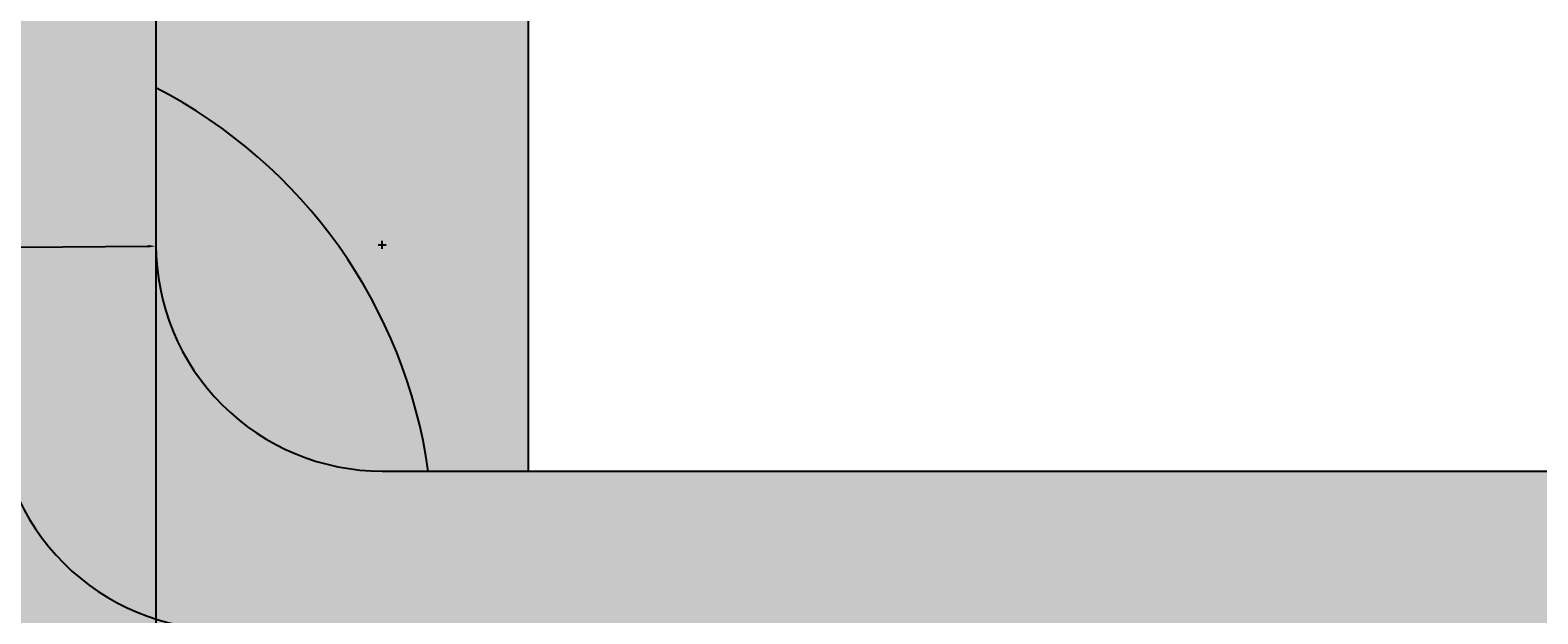
# Model space of a CAD drawing. Units: millimetres. Extents: x -11 to 280, y -4 to 208.
# Tile 33 of 55: x 189 to 222, y 76 to 88. Entities that reach past the tile are written whole.
import ezdxf

# ---------------------------------------------------------------- set-up
doc = ezdxf.new("R2010")
doc.units = ezdxf.units.MM
for name, color, linetype, lineweight in [('M-DIMS', 2, 'Continuous', 18), ('M-HYDR-PRES', 7, 'Continuous', 25), ('M-HYDR-VALV', 7, 'Continuous', 25), ('M-HYDR-VALV-PATT', 252, 'Continuous', 13)]:
    doc.layers.add(name, color=color, linetype=linetype, lineweight=lineweight)
doc.layers.add('M-HYDR-PRES-PATT', color=240, linetype='Continuous', lineweight=13, true_color=0xed1f24)
doc.styles.get("Standard").update_dxf_attribs({"font": 'arial.ttf'})
doc.dimstyles.get("Standard").update_dxf_attribs({"dimtxt": 0.18, "dimasz": 0.18, "dimexe": 0.18, "dimexo": 0.0625, "dimgap": 0.09, "dimtad": 0, "dimtih": 1, "dimtoh": 1, "dimdec": 4, "dimzin": 0, "dimdsep": 46, "dimtxsty": 'Standard', "dimcen": 0.09, "dimadec": 0, "dimazin": 0, "dimtfac": 1, "dimtdec": 4, "dimtofl": 0, "dimtmove": 0, "dimatfit": 3, "dimfxl": 1, "dimtolj": 1, "dimtzin": 0, "dimarcsym": 0})

# ---------------------------------------------------------------- blocks, each defined once
blk = doc.blocks.new('*D4')
at = {"layer": 'Defpoints', "color": 0, "transparency": 16777216}
for p in [(4.763, 84.426), (266.035, 51.733), (266.035, -3.415)]:
    blk.add_point(p, dxfattribs=at)
at = {"layer": 'M-DIMS', "color": 0, "lineweight": -2, "transparency": 16777216}
for p, q in [((4.763, 84.364), (4.763, -3.595)), ((266.035, 51.67), (266.035, -3.595)), ((4.943, -3.415), (134.934, -3.415)), ((265.855, -3.415), (135.864, -3.415))]:
    blk.add_line(p, q, dxfattribs=at)
at = {"layer": 'M-DIMS', "color": 0, "transparency": 16777216}
for points in [[(4.943, -3.385), (4.943, -3.445), (4.763, -3.415)], [(265.855, -3.385), (265.855, -3.445), (266.035, -3.415)]]:
    blk.add_solid(points, dxfattribs=at)
at = {"layer": 'M-DIMS', "color": 0, "transparency": 16777216, "insert": (135.399, -3.415), "char_height": 0.18, "attachment_point": 5}
blk.add_mtext('\\A1;261.27', dxfattribs=at)
blk = doc.blocks.new('*D5')
at = {"layer": 'Defpoints', "color": 0, "transparency": 16777216}
for p in [(24.759, 192.645), (-10.087, 11.435), (261.686, 11.435)]:
    blk.add_point(p, dxfattribs=at)
at = {"layer": 'M-DIMS', "color": 0, "lineweight": -2, "transparency": 16777216}
for p, q in [((24.696, 192.645), (-10.267, 192.645)), ((-10.087, 192.465), (-10.087, 102.222)), ((-10.087, 11.615), (-10.087, 101.858)), ((261.624, 11.435), (-10.267, 11.435))]:
    blk.add_line(p, q, dxfattribs=at)
at = {"layer": 'M-DIMS', "color": 0, "transparency": 16777216}
for points in [[(-10.117, 192.465), (-10.057, 192.465), (-10.087, 192.645)], [(-10.117, 11.615), (-10.057, 11.615), (-10.087, 11.435)]]:
    blk.add_solid(points, dxfattribs=at)
at = {"layer": 'M-DIMS', "color": 0, "transparency": 16777216, "insert": (-10.087, 102.04), "char_height": 0.18, "attachment_point": 5}
blk.add_mtext('\\A1;181.2', dxfattribs=at)
blk = doc.blocks.new('*D13')
at = {"layer": 'Defpoints', "color": 0, "transparency": 16777216}
for p in [(191.774, 105.314), (232.2, 105.314), (232.2, -3.415)]:
    blk.add_point(p, dxfattribs=at)
at = {"layer": 'M-DIMS', "color": 0, "lineweight": -2, "transparency": 16777216}
for p, q in [((191.774, 105.252), (191.774, -3.595)), ((232.2, 105.252), (232.2, -3.595)), ((191.954, -3.415), (211.52, -3.415)), ((232.02, -3.415), (212.454, -3.415))]:
    blk.add_line(p, q, dxfattribs=at)
at = {"layer": 'M-DIMS', "color": 0, "transparency": 16777216}
for points in [[(191.954, -3.385), (191.954, -3.445), (191.774, -3.415)], [(232.02, -3.385), (232.02, -3.445), (232.2, -3.415)]]:
    blk.add_solid(points, dxfattribs=at)
at = {"layer": 'M-DIMS', "color": 0, "transparency": 16777216, "insert": (211.987, -3.415), "char_height": 0.18, "attachment_point": 5}
blk.add_mtext('\\A1;40.426', dxfattribs=at)
blk = doc.blocks.new('*D20')
at = {"layer": 'Defpoints', "color": 0, "transparency": 16777216}
for p in [(231.68, 207.495), (151.022, 43.599), (231.68, 43.599)]:
    blk.add_point(p, dxfattribs=at)
at = {"layer": 'M-DIMS', "color": 0, "lineweight": -2, "transparency": 16777216}
for p, q in [((151.022, 43.662), (151.022, 207.675)), ((231.68, 43.662), (231.68, 207.675)), ((151.202, 207.495), (190.957, 207.495)), ((231.5, 207.495), (191.745, 207.495))]:
    blk.add_line(p, q, dxfattribs=at)
at = {"layer": 'M-DIMS', "color": 0, "transparency": 16777216}
for points in [[(151.202, 207.525), (151.202, 207.465), (151.022, 207.495)], [(231.5, 207.525), (231.5, 207.465), (231.68, 207.495)]]:
    blk.add_solid(points, dxfattribs=at)
at = {"layer": 'M-DIMS', "color": 0, "transparency": 16777216, "insert": (191.351, 207.495), "char_height": 0.18, "attachment_point": 5}
blk.add_mtext('\\A1;80.66', dxfattribs=at)
blk = doc.blocks.new('*D31')
at = {"layer": 'Defpoints', "color": 0, "transparency": 16777216}
for p in [(191.775, 83.68), (196.774, 83.71)]:
    blk.add_point(p, dxfattribs=at)
at = {"layer": 'M-DIMS', "color": 0, "lineweight": -2, "transparency": 16777216}
for p, q in [((188.775, 83.662), (191.595, 83.679)), ((196.684, 83.71), (196.864, 83.71)), ((196.774, 83.62), (196.774, 83.8))]:
    blk.add_line(p, q, dxfattribs=at)
at = {"layer": 'M-DIMS', "color": 0, "transparency": 16777216}
blk.add_solid([(191.594, 83.709), (191.595, 83.649), (191.775, 83.68)], dxfattribs=at)
at = {"layer": 'M-DIMS', "color": 0, "transparency": 16777216, "insert": (188.342, 83.662), "char_height": 0.18, "attachment_point": 5}
blk.add_mtext('\\A1;4X R5', dxfattribs=at)

msp = doc.modelspace()

# ---------------------------------------------------------------- hatches: boundary and pattern name
at = {"layer": 'M-HYDR-PRES-PATT'}
h = msp.add_hatch(color=256, dxfattribs=at)
h.set_gradient(color1=(237, 31, 36), color2=(237, 31, 36), tint=1)
h.paths.add_polyline_path([(232.2, 133.1228), (228.7, 133.1228), (228.7, 108.8141), (102.7646, 108.8141), (102.7646, 105.3141), (232.2, 105.3141)])
h.paths.add_polyline_path([(128.8433, 105.3141), (125.3433, 105.3141), (125.3433, 91.7099, 1), (128.8433, 91.7099)])
h.paths.add_polyline_path([(229.1617, 78.7098), (196.7745, 78.7098, -0.4142136), (191.7745, 83.7098), (191.7745, 105.3141), (188.2745, 105.3141), (188.2745, 80.2098, 0.4142136), (193.2745, 75.2098), (225.6617, 75.2098), (225.6617, 43.5991), (229.1617, 43.5991)])
h.paths.add_polyline_path([(102.7646, 110.3704), (95.5776, 110.3704), (95.5776, 103.9022), (102.7646, 103.9022)])
h.paths.add_polyline_path([(100.7059, 107.2502), (99.1711, 106.3641), (99.1711, 106.8641), (97.1711, 106.8641), (97.1711, 107.6363), (99.1711, 107.6363), (99.1711, 108.1363)], flags=16)
h.paths.add_polyline_path([(234.6119, 138.4081), (226.5106, 138.4081), (226.5106, 133.1228), (234.6119, 133.1228)])
h.paths.add_polyline_path([(231.1963, 135.7055), (230.2965, 134.1786), (229.4241, 135.7213), (229.9241, 135.7168), (229.9418, 137.7167), (230.7141, 137.7099), (230.6963, 135.71)], flags=16)
at = {"layer": 'M-HYDR-VALV-PATT'}
h = msp.add_hatch(color=256, dxfattribs=at)
h.set_gradient(color1=(153, 27, 30), color2=(153, 27, 30), tint=1)
h.paths.add_polyline_path([(131.8437, 88.2421, -0.3394543), (132.5849, 89.208), (121.2548, 86.1721, -0.4931454), (122.5137, 85.2062, -0.3394543), (121.7725, 84.2403), (133.1025, 87.2762, -0.4931454)])
h.paths.add_polyline_path([(133.1025, 83.1351, -0.4931454), (131.8437, 84.101, -0.3394543), (132.5849, 85.0669), (121.2548, 82.031, -0.4931454), (122.5137, 81.0651, -0.3394543), (121.7725, 80.0992)])
h.paths.add_polyline_path([(133.1025, 78.994, -0.4931454), (131.8437, 79.9599, -0.3394543), (132.5849, 80.9258), (121.2548, 77.8899, -0.4931454), (122.5137, 76.924, -0.3394543), (121.7725, 75.9581)])
h.paths.add_polyline_path([(197.7905, 78.7098), (200.0003, 78.7098), (200.0003, 89.3873), (191.7745, 89.3873), (191.7745, 87.1776, -0.2439164)])
h.paths.add_polyline_path([(200.0003, 65.0638), (200.0003, 75.2098), (197.7325, 75.2098, -0.4135811), (184.7092, 66.0277), (184.7092, 65.0638)])
h.paths.add_polyline_path([(181.2092, 65.0638), (181.2092, 67.2471, -0.2598454), (175.3563, 76.54), (173.8038, 76.54), (173.8038, 65.0638)])
h.paths.add_polyline_path([(188.2745, 88.3022), (188.2745, 89.3873), (173.8038, 89.3873), (173.8038, 80.04), (175.7181, 80.04, -0.3816661)])
h = msp.add_hatch(color=256, dxfattribs=at)
h.set_gradient(color1=(205, 105, 40), color2=(34, 52, 110), tint=1, name='INVCYLINDER')
h.paths.add_polyline_path([(188.2745, 80.2098), (188.2745, 88.3022, 0.3816661), (175.7181, 80.04), (179.7092, 80.04, -0.4142136), (184.7092, 75.04), (184.7092, 66.0277, 0.4135811), (197.7325, 75.2098), (193.2745, 75.2098, -0.4142136)])
h.paths.add_polyline_path([(176.2092, 76.54), (175.3563, 76.54, 0.2598454), (181.2092, 67.2471), (181.2092, 71.54, 0.4142136)])
h.paths.add_polyline_path([(196.7745, 78.7098), (197.7905, 78.7098, 0.2439164), (191.7745, 87.1776), (191.7745, 83.7098, 0.4142136)])

# ---------------------------------------------------------------- linework, layer by layer
at = {"layer": 'M-HYDR-PRES'}
for points in [[(188.2745, 105.3141), (188.2745, 80.2098, 0.4142136), (193.2745, 75.2098), (225.6617, 75.2098), (225.6617, 43.5991)], [(191.7745, 105.3141), (191.7745, 83.7098, 0.4142136), (196.7745, 78.7098), (229.1617, 78.7098), (229.1617, 43.5991)]]:
    msp.add_lwpolyline(points, format="xyb", dxfattribs=at)
at = {"layer": 'M-HYDR-VALV'}
msp.add_lwpolyline([(191.7745, 89.3873), (200.0003, 89.3873), (200.0003, 78.7098)], dxfattribs=at)
msp.add_arc((186.6199, 77.1445), 11.2798, 7.9769, 62.80777, dxfattribs=at)

# ---------------------------------------------------------------- dimensions: what is measured, and where the dimension line sits
at = {"layer": 'M-DIMS'}
for base, p1, p2, override, picture, middle in [((231.6803, 207.495), (151.0217, 43.5991), (231.6803, 43.5991), {"dimdec": 2, "dimlfac": 1, "dimrnd": 0, "dimzin": 0, "dimdsep": 46, "dimlunit": 2}, '*D20', (191.351, 207.495)), ((232.20002, -3.41542), (191.77448, 105.31407), (232.20002, 105.31407), {"dimdec": 3, "dimlfac": 1, "dimrnd": 0, "dimzin": 0, "dimdsep": 46, "dimlunit": 2}, '*D13', (211.98725, -3.41542)), ((266.0352, -3.4154), (4.7635, 84.4261), (266.0352, 51.7328), {"dimdec": 2, "dimlfac": 1, "dimrnd": 0, "dimzin": 0, "dimdsep": 46, "dimlunit": 2}, '*D4', (135.3993, -3.4154))]:
    dim = msp.add_linear_dim(base=base, p1=p1, p2=p2, dimstyle='Standard', override=override, dxfattribs=at)
    dim.commit()
    dim.dimension.update_dxf_attribs({"geometry": picture, "text_midpoint": middle})
dim = msp.add_linear_dim(base=(-10.0865, 11.4346), p1=(24.7588, 192.645), p2=(261.6863, 11.4346), angle=90, dimstyle='Standard', override={"dimdec": 1, "dimlfac": 1, "dimrnd": 0, "dimzin": 0, "dimdsep": 46, "dimlunit": 2}, dxfattribs=at)
dim.commit()
dim.dimension.update_dxf_attribs({"geometry": '*D5', "text_midpoint": (-10.0865, 102.0398)})
dim = msp.add_radius_dim(center=(196.7745, 83.7098), mpoint=(191.7746, 83.6801), text='4X <>', dimstyle='Standard', override={"dimdec": 0, "dimlfac": 1, "dimrnd": 0, "dimzin": 0, "dimdsep": 46, "dimlunit": 2}, dxfattribs=at)
dim.commit()
dim.dimension.update_dxf_attribs({"geometry": '*D31', "text_midpoint": (188.7746, 83.6623), "dimtype": 164})

doc.saveas('drawing.dxf')
